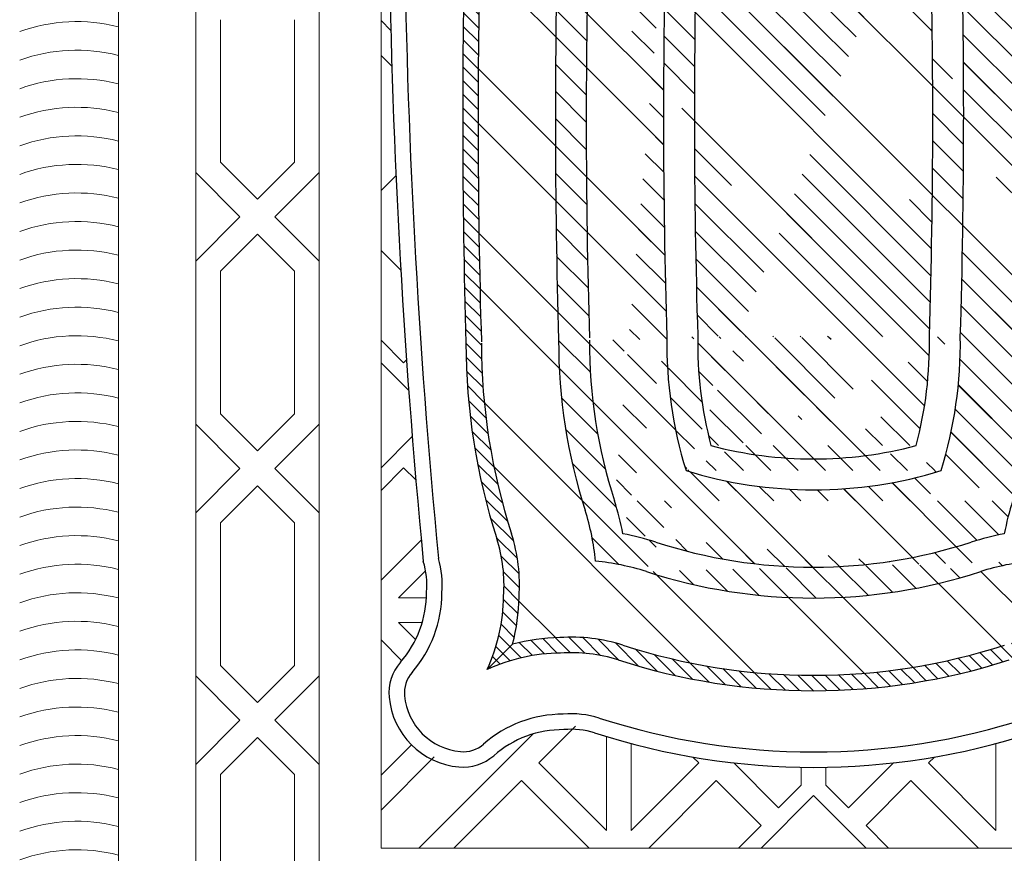
# Model space of a CAD drawing. Units: inches. Extents: x 3592 to 4861, y 1650 to 2243.
# Tile 7 of 30: x 4188 to 4207, y 1916 to 1932. Entities that reach past the tile are written whole.
import ezdxf

# ---------------------------------------------------------------- set-up
doc = ezdxf.new("R2010")
doc.units = ezdxf.units.IN
doc.layers.add('A-FURN', color=9, linetype='Continuous', lineweight=13)
doc.layers.add('RA-AP-01$0$INT', color=35, linetype='Continuous', lineweight=5)
for name, color, linetype in [('RA-AP-01$0$FURN', 3, 'Continuous'), ('RA-AP-01$0$WOOD', 64, 'Continuous'), ('RA-AP-02$0$FLPT', 30, 'Continuous')]:
    doc.layers.add(name, color=color, linetype=linetype)

# ---------------------------------------------------------------- blocks, each defined once
blk = doc.blocks.new('A$C67D63ADA')
at = {"layer": 'RA-AP-01$0$INT'}
for p, q in [((5.477240000007288, -6.923416270324413), (5.477239999992479, -6.363416270332882)), ((5.409652332498168, -6.525357395822982), (5.465926291497726, -6.525357395821494)), ((5.465926291497726, -6.525357395821494), (5.42221056274693, -6.569073124574231)), ((5.477239999997057, -6.536671104320128), (5.433524271246167, -6.580386833072967)), ((5.477239999998595, -6.59484772782809), (5.477239999997057, -6.536671104320128)), ((5.418357259801259, -6.565219821628732), (5.42221056274693, -6.569073124574231)), ((5.433524271246167, -6.580386833072966), (5.462612583000919, -6.609475144826422)), ((5.422140622500873, -6.591770481818769), (5.422210562747435, -6.591700541572205)), ((5.422210562747434, -6.591700541572205), (5.451298874502183, -6.62078885332566)), ((5.462612583000919, -6.609475144826422), (5.477239999998558, -6.594847727828128)), ((5.477239999998596, -6.59484772782809), (5.462612583000919, -6.609475144826423)), ((5.443298874502688, -6.64341627032368), (5.477239999998885, -6.609475144825973)), ((5.477239999998885, -6.609475144825973), (5.477240000000778, -6.677357395819498)), ((5.43667145750578, -6.635416270323993), (5.451298874503459, -6.620788853325663)), ((5.436671457504505, -6.635416270323988), (5.424977006995209, -6.635416270324199)), ((5.443298874502688, -6.64341627032368), (5.477240000000778, -6.677357395819498)), ((5.436671457504861, -6.651416270322137), (5.424977006995124, -6.651416270322447)), ((5.436671457506382, -6.65141627032399), (5.451298874503189, -6.666043687319815)), ((5.422210562749734, -6.695131999074563), (5.451298874503189, -6.666043687319815)), ((5.433524271248971, -6.706445707574319), (5.462612583002428, -6.677357395819569)), ((5.477240000000758, -6.691984812817247), (5.462612583002428, -6.677357395819567)), ((5.477240000000756, -6.691984812817247), (5.477240000001805, -6.750161436325209)), ((5.422140622500601, -6.695062058825432), (5.422210562749736, -6.695131999074563)), ((5.477240000001805, -6.750161436325209), (5.433524271248971, -6.706445707574317)), ((5.41835725979925, -6.721612719024712), (5.422210562750238, -6.717759416073553)), ((5.465926291502978, -6.761475144824349), (5.422210562750238, -6.717759416073553)), ((5.409652332496428, -6.761475144825365), (5.465926291502978, -6.761475144824349)), ((5.405096589281656, -6.777475144825446), (5.465926291503357, -6.777475144824348)), ((5.465926291503357, -6.777475144824348), (5.422210562752948, -6.821190873576702)), ((5.477240000002503, -6.788788853323175), (5.433524271252185, -6.832504582075438)), ((5.422210562752947, -6.821190873576701), (5.398502923497431, -6.797483234322237)), ((5.403480564853991, -6.825088292684419), (5.477240000004493, -6.898847727834922)), ((5.477240000004083, -6.876220310825392), (5.433524271252185, -6.832504582075438)), ((5.418311572313375, -6.889056385133678), (5.452671457504211, -6.923416270324519)), ((5.315298874504621, -6.912102561826071), (5.29779276232685, -6.894596449648303)), ((5.315298874504541, -6.893742340800933), (5.315298874504621, -6.912102561826071)), ((5.239087008341665, -6.900882970485501), (5.231181125499767, -6.908788853327399)), ((5.303985166005732, -6.923416270325152), (5.277960454425306, -6.89739155874473)), ((5.331298874504555, -6.896756776930311), (5.33129887450462, -6.912102561826093)), ((5.33129887450462, -6.912102561826093), (5.342348500618869, -6.901052935711843)), ((5.148671457508614, -6.923416270325409), (5.16329887450662, -6.908788853327405)), ((5.163298874506619, -6.908788853327405), (5.148671457508651, -6.923416270325372)), ((5.161430071025033, -6.906920049845819), (5.163298874506619, -6.908788853327405)), ((5.181214712172991, -6.905500432658874), (5.163298874506496, -6.923416270325372)), ((5.210977238572697, -6.903212383397972), (5.231181125500023, -6.923416270325749)), ((5.245808542497771, -6.923416270325402), (5.231181125499765, -6.908788853327399)), ((5.430044040505915, -6.923416270324613), (5.410388987144851, -6.903761216963554)), ((5.051867417002686, -6.92341627032501), (5.042215760114743, -6.913764613437067)), ((5.079181125501765, -6.912102561826092), (5.079336333743704, -6.911947353584153)), ((5.079181125501766, -6.911955542479179), (5.079181125501765, -6.912102561826092)), ((5.090494834000653, -6.923416270325169), (5.103286866518899, -6.91062423780692)), ((5.3426125830037, -6.923416270324986), (5.356067157599694, -6.909961695728989)), ((4.948123212422537, -6.917101600404618), (4.941808542500447, -6.923416270326709)), ((4.964435959500471, -6.923416270324652), (4.971407022751201, -6.916445207073921)), ((4.877240000006825, -6.923416270326986), (5.477240000007288, -6.923416270324413)), ((5.051867417002687, -6.923416270325013), (4.964435959500471, -6.923416270324652)), ((5.148671457508614, -6.923416270325408), (5.090494834000653, -6.923416270325169)), ((5.163298874506496, -6.923416270325372), (5.231181125500023, -6.923416270325749)), ((5.245808542497771, -6.923416270325401), (5.303985166005732, -6.923416270325152)), ((5.040068427124683, -6.963416270301689), (5.068754718630654, -6.992102561798438)), ((5.097441010136626, -6.963416270301689), (5.068754718630654, -6.992102561798438)), ((5.202896854259693, -6.963416270316853), (5.231583145756439, -6.992102561822827)), ((5.260269437262412, -6.963416270301053), (5.23158314575644, -6.992102561797802)), ((5.36572528138184, -6.963416270321417), (5.394411572878586, -6.99210256182739)), ((5.394411572878586, -6.99210256182739), (5.423097864384927, -6.963416270330275)), ((5.033441010127117, -6.979416270300584), (4.941240000005749, -6.979416270315998)), ((5.033441010127117, -6.979416270300584), (5.057441010133491, -7.00341627029924)), ((5.104068427130107, -6.979416270304665), (5.080068427127819, -7.00341627029924)), ((5.104068427130107, -6.979416270304665), (5.196269437263445, -6.979416270320077)), ((5.196269437263445, -6.979416270320077), (5.220269437255637, -7.003416270319991)), ((5.266896854262809, -6.979416270297111), (5.242896854253604, -7.003416270298604)), ((5.266896854262809, -6.979416270297111), (5.359097864373478, -6.979416270312523)), ((5.359097864373478, -6.979416270312523), (5.383097864377784, -7.003416270324554)), ((5.405725281375753, -7.003416270328198), (5.42972528138643, -6.979416270325234)), ((5.52192629150337, -6.97941627032422), (5.42972528138643, -6.979416270325234)), ((5.033441010139864, -7.027416270300586), (5.057441010133491, -7.00341627029924)), ((5.104068427125523, -7.027416270304664), (5.080068427127819, -7.00341627029924)), ((5.196269437247836, -7.027416270320077), (5.220269437255637, -7.003416270319991)), ((5.266896854244392, -7.027416270297113), (5.242896854253604, -7.003416270298604)), ((5.359097864382099, -7.027416270312525), (5.383097864377784, -7.003416270324554)), ((5.405725281375753, -7.003416270328198), (5.429725281365354, -7.027416270325517)), ((5.040068427138238, -7.043416270301689), (5.068754718634292, -7.014729978796407)), ((5.097441010123072, -7.043416270301689), (5.068754718627016, -7.014729978796407)), ((5.202896854247523, -7.043416270316853), (5.231583145752804, -7.014729978820797)), ((5.260269437248857, -7.043416270301053), (5.231583145752802, -7.01472997879577)), ((5.36572528136967, -7.043416270321417), (5.394411572874951, -7.014729978825361)), ((5.394411572874951, -7.014729978825361), (5.423097864372064, -7.043416270331702)), ((5.033441010139864, -7.027416270300586), (4.941240000013775, -7.027416270315999)), ((5.104068427125523, -7.027416270304664), (5.196269437247836, -7.027416270320077)), ((5.266896854244392, -7.027416270297113), (5.359097864382099, -7.027416270312525)), ((5.429725281365354, -7.027416270325517), (5.521926291510647, -7.027416270325517))]:
    blk.add_line(p, q, dxfattribs=at)
for points in [[(5.647240000006826, -6.243416270325369), (5.647240000006826, -7.09341627032537), (4.107240000006826, -7.093416270325372), (4.107240000006826, -6.19341627032537), (4.877240000006826, -6.19341627032537)], [(4.877240000006826, -6.19341627032537), (5.647240000006826, -6.19341627032537), (5.647240000006826, -7.09341627032537), (4.877240000006826, -7.09341627032537)], [(5.597240000006826, -6.243416270325369), (5.597240000006826, -7.04341627032537), (4.157240000006826, -7.043416270325372), (4.157240000006826, -6.243416270325369)], [(4.877240000006826, -6.32341627032537), (5.517240000006826, -6.32341627032537), (5.517240000006826, -6.963416270325371), (4.877240000006826, -6.963416270325371)]]:
    blk.add_lwpolyline(points, dxfattribs=at)
for centre, start in [((5.051601958963728, -7.120376270327977), 165.6974573627986), ((5.070081958960181, -7.120376270327977), 165.6974573627986), ((5.088561958964091, -7.120376270329249), 165.6974573621089), ((5.10704195896309, -7.120376270327067), 165.6974573632914), ((5.12552195896209, -7.120376270327067), 165.6974573632914), ((5.144001958965818, -7.12037627032834), 165.6974573626017), ((5.162481958964817, -7.12037627032743), 165.6974573630946), ((5.18096195896127, -7.12037627032743), 165.6974573630946), ((5.19944195896518, -7.120376270328703), 165.6974573624049), ((5.217921958963997, -7.120376270330159), 165.6974573616162), ((5.236401958960631, -7.120376270327794), 165.6974573628977), ((5.25488195896436, -7.120376270327977), 165.6974573627986), ((5.273361958963359, -7.120376270329249), 165.6974573621089), ((5.291841958964723, -7.120376270330522), 165.6974573614194), ((5.310321958963722, -7.12037627032834), 165.6974573626017), ((5.328801958964235, -7.120376270330886), 165.6974573612222), ((5.328801958965086, -7.120376270328522), 165.6974573625031), ((5.347281958963233, -7.120376270328703), 165.6974573624049), ((5.365761958962233, -7.120376270328703), 165.6974573624049), ((5.384241958965962, -7.120376270329977), 165.6974573617145), ((5.402721958964961, -7.120376270329067), 165.6974573622072), ((5.421201958961413, -7.120376270329067), 165.6974573622072), ((5.439681958965324, -7.120376270330341), 165.6974573615171), ((5.458161958964141, -7.120376270331796), 165.6974573607288), ((5.476641958960775, -7.120376270329431), 165.6974573620099), ((5.495121958964504, -7.120376270329613), 165.6974573619117), ((5.513601958963502, -7.120376270330886), 165.6974573612216), ((5.532081958964867, -7.12037627033216), 165.6974573605316), ((5.550561958963865, -7.120376270329977), 165.6974573617144), ((5.56904195896523, -7.120376270330159), 165.6974573616157), ((5.587521958961682, -7.120376270332524), 165.6974573603342)]:
    blk.add_arc(centre, 0.1091312342836184, start, 199.7961568705686, dxfattribs=at)
blk = doc.blocks.new('A$C09A87C41')
at = {"layer": 'RA-AP-01$0$WOOD'}
h = blk.add_hatch(dxfattribs=at)
h.set_pattern_fill('ANSI31', color=256, scale=0.05, style=0)
h.set_pattern_definition([(45, (0.7182879904584168, -11.54818755465011), (0.0044194173824159, -0.0044194173824159), [])])
edge = h.paths.add_edge_path()
edge.add_ellipse((5.006516613079209, -11.27459283286495), major_axis=(3.435359877543153, 3.435359877543153), ratio=0.9999999999999982, start_angle=403.3022422558093, end_angle=406.5486575131389, ccw=False)
edge.add_ellipse((5.150455045735207, -6.828790194879051), major_axis=(-0.2901946312779826, 0.2901946312779826), ratio=0.9999999999999875, start_angle=297.2093186994243, end_angle=314.9999999999731, ccw=False)
edge.add_ellipse((5.307117976013378, -6.343033378039902), major_axis=(-0.0707106781186454, 0.0707106781186455), ratio=0.9999999999999651, start_angle=116.7779839927149, end_angle=139.0873288843009)
edge.add_ellipse((5.312718414970339, -6.324818905441738), major_axis=(0.0834173982641243, 0.0834173982641243), ratio=0.9999999999999847, start_angle=225.741775187377, end_angle=249.5633269497028)
edge.add_line((5.361758401537698, -6.432112914518591), (5.345299417747169, -6.448571898309089))
edge.add_ellipse((5.312718414970311, -6.32481890544173), major_axis=(-0.0904884660759946, 0.0904884660759945), ratio=0.9999999999999644, start_angle=135.8720682536374, end_angle=149.7498089726665, ccw=False)
edge.add_ellipse((5.307117976013483, -6.343033378039922), major_axis=(-0.0777817459304867, 0.0777817459304867), ratio=0.9999999999999941, start_angle=117.45144083316339, end_angle=138.9346900893823, ccw=False)
edge.add_ellipse((5.150455045735208, -6.82879019487905), major_axis=(0.2831235634661059, 0.2831235634661059), ratio=0.9999999999999859, start_angle=27.03507540014952, end_angle=44.9867285887044)
edge.add_ellipse((5.006516315412802, -11.27459997798134), major_axis=(-3.428298916554014, 3.428298916554014), ratio=0.9999999999999971, start_angle=-46.70235550375367, end_angle=-43.44815559494434)
edge.add_ellipse((4.743915471599394, -11.2745999779814), major_axis=(3.428298916553931, 3.42829891655393), ratio=0.9999999999999994, start_angle=43.44815559494427, end_angle=46.70235550375375)
edge.add_ellipse((4.599976741276995, -6.828790194879051), major_axis=(0.2831235634661173, 0.2831235634661172), ratio=0.9999999999999861, start_angle=45.01327141129749, end_angle=62.96492459984043)
edge.add_ellipse((4.443313810998718, -6.343033378039922), major_axis=(0.0777817459304893, 0.0777817459304893), ratio=0.9999999999999873, start_angle=221.0653099106178, end_angle=242.54855916687399, ccw=False)
edge.add_ellipse((4.437713372041892, -6.32481890544173), major_axis=(0.0904884660759951, 0.0904884660759951), ratio=0.9999999999999603, start_angle=210.2501910273332, end_angle=224.1279317463614, ccw=False)
edge.add_line((4.405132369265034, -6.448571898309089), (4.388673385474508, -6.432112914518594))
edge.add_ellipse((4.43771337204186, -6.324818905441737), major_axis=(0.0834173982641232, 0.0834173982641232), ratio=0.9999999999999797, start_angle=200.4366730503009, end_angle=224.2582248126243)
edge.add_ellipse((4.443313810998827, -6.343033378039902), major_axis=(-0.0707106781186382, 0.0707106781186382), ratio=0.9999999999999952, start_angle=130.9126711156974, end_angle=153.2220160072772)
edge.add_ellipse((4.599976741276995, -6.828790194879051), major_axis=(-0.2901946312779718, 0.2901946312779718), ratio=0.9999999999999895, start_angle=315.0000000000233, end_angle=332.7906813005773, ccw=False)
edge.add_ellipse((4.743915173933024, -11.27459283286497), major_axis=(-3.435359877543123, 3.435359877543123), ratio=0.9999999999999991, start_angle=313.451342486861, end_angle=316.69775774419077, ccw=False)
edge = h.paths.add_edge_path()
edge.add_ellipse((4.299593848995801, -6.48675334004306), major_axis=(-0.0707106781186556, 0.0707106781186556), ratio=0.9999999999999859, start_angle=206.7779839906583, end_angle=229.0873288838364)
edge.add_ellipse((4.281379376397651, -6.481152901086075), major_axis=(-0.0834173982641623, 0.0834173982641623), ratio=0.9999999999999754, start_angle=225.7417751869729, end_angle=249.5633269497573)
edge.add_line((4.388673385474506, -6.432112914518592), (4.405132369265034, -6.448571898309089))
edge.add_ellipse((4.281379376397657, -6.481152901086004), major_axis=(-0.0904884660760182, 0.0904884660760182), ratio=0.9999999999999957, start_angle=225.8720682533453, end_angle=239.7498089726896, ccw=False)
edge.add_ellipse((4.299593848995796, -6.486753340043026), major_axis=(0.0777817459305317, 0.0777817459305317), ratio=0.9999999999999891, start_angle=297.4514408381613, end_angle=318.9346900891407, ccw=False)
edge.add_ellipse((4.785350665835052, -6.643416270320893), major_axis=(0.2831235634661102, 0.2831235634661102), ratio=0.9999999999999978, start_angle=117.0350753988375, end_angle=152.9649246009711)
edge.add_ellipse((4.299593848995777, -6.800079200598784), major_axis=(-0.0777817459305426, 0.0777817459305426), ratio=0.9999999999999973, start_angle=221.0653099111909, end_angle=242.5485591625442, ccw=False)
edge.add_ellipse((4.281379376397679, -6.805679639555494), major_axis=(-0.0904884660760244, 0.0904884660760244), ratio=0.9999999999999076, start_angle=210.2501910270576, end_angle=224.1279317467988, ccw=False)
edge.add_line((4.405132369264926, -6.838260642332959), (4.388673385474263, -6.854719626123697))
edge.add_ellipse((4.281379376397679, -6.80567963955562), major_axis=(0.0834173982641642, 0.0834173982641642), ratio=0.9999999999999609, start_angle=290.4366730499258, end_angle=314.2582248131156)
edge.add_ellipse((4.299593848995804, -6.800079200598786), major_axis=(-0.0707106781186612, 0.0707106781186612), ratio=0.999999999999977, start_angle=220.9126711163551, end_angle=243.222016008517)
edge.add_ellipse((4.785350665835053, -6.643416270320894), major_axis=(0.2901946312779783, 0.2901946312779783), ratio=0.9999999999999984, start_angle=117.2093186999746, end_angle=152.7906813002342, ccw=False)
edge = h.paths.add_edge_path()
edge.add_ellipse((4.743915471599392, -2.012232562660299), major_axis=(3.428298916553894, 3.428298916553894), ratio=0.9999999999999992, start_angle=223.2976444962459, end_angle=226.5518444050561)
edge.add_ellipse((5.006516315412771, -2.012232562660296), major_axis=(3.428298916553752, 3.428298916553752), ratio=0.9999999999999971, start_angle=223.448155594945, end_angle=226.7023555037531)
edge.add_ellipse((5.150455045735209, -6.458042345762599), major_axis=(0.283123563466111, 0.283123563466111), ratio=0.999999999999996, start_angle=225.0132714112834, end_angle=242.9649246011241)
edge.add_ellipse((5.30711797601273, -6.94379916260194), major_axis=(0.0777817459305174, 0.0777817459305174), ratio=0.9999999999999873, start_angle=401.06530991071423, end_angle=422.548559161793, ccw=False)
edge.add_ellipse((5.312718414969516, -6.962013635200094), major_axis=(0.0904884660760023, 0.0904884660760023), ratio=0.9999999999999566, start_angle=390.2501910269164, end_angle=404.12793174642553, ccw=False)
edge.add_line((5.345299417747278, -6.838260642332959), (5.361758401537942, -6.854719626123698))
edge.add_ellipse((5.312718414969516, -6.962013635200098), major_axis=(0.0834173982641439, 0.0834173982641439), ratio=0.9999999999999785, start_angle=20.43667304973462, end_angle=44.25822481258737)
edge.add_ellipse((5.307117976012772, -6.943799162601948), major_axis=(-0.0707106781186618, 0.0707106781186618), ratio=0.999999999999977, start_angle=-49.08732888421749, end_angle=-26.77798399064677)
edge.add_ellipse((5.150455045735209, -6.458042345762597), major_axis=(0.2901946312779783, 0.2901946312779783), ratio=0.9999999999999957, start_angle=225.0000000000273, end_angle=242.7906812999824, ccw=False)
edge.add_ellipse((5.006516613079198, -2.012239707776725), major_axis=(3.43535987754352, 3.43535987754352), ratio=0.999999999999996, start_angle=223.4513424868609, end_angle=226.697757744191, ccw=False)
edge.add_ellipse((4.743915173933023, -2.012239707776712), major_axis=(3.435359877543229, 3.435359877543229), ratio=0.9999999999999998, start_angle=223.3022422558095, end_angle=226.5486575131387, ccw=False)
edge.add_ellipse((4.599976741276995, -6.458042345762597), major_axis=(0.2901946312779746, 0.2901946312779748), ratio=0.9999999999999964, start_angle=207.2093187000184, end_angle=224.9999999999795, ccw=False)
edge.add_ellipse((4.443313810999427, -6.943799162601947), major_axis=(-0.070710678118668, 0.070710678118668), ratio=0.9999999999999838, start_angle=-63.22201600935903, end_angle=-40.9126711157662)
edge.add_ellipse((4.437713372042683, -6.962013635200099), major_axis=(0.0834173982641484, 0.0834173982641484), ratio=0.9999999999999729, start_angle=45.74177518742643, end_angle=69.56332695026246)
edge.add_line((4.388673385474263, -6.854719626123697), (4.405132369264926, -6.838260642332958))
edge.add_ellipse((4.437713372042681, -6.962013635200094), major_axis=(0.0904884660760224, 0.0904884660760225), ratio=0.9999999999999282, start_angle=405.87206825357924, end_angle=419.7498089730807, ccw=False)
edge.add_ellipse((4.443313810999475, -6.94379916260194), major_axis=(-0.0777817459305165, 0.0777817459305165), ratio=0.9999999999999927, start_angle=297.4514408382556, end_angle=318.93469008929503, ccw=False)
edge.add_ellipse((4.599976741276995, -6.458042345762597), major_axis=(0.2831235634661077, 0.2831235634661077), ratio=0.9999999999999937, start_angle=207.0350753988627, end_angle=224.9867285886981)
edge = h.paths.add_edge_path()
edge.add_ellipse((5.450837938016399, -6.800079200598789), major_axis=(-0.0707106781186565, 0.0707106781186565), ratio=0.9999999999999875, start_angle=26.77798399147072, end_angle=49.08732888364846)
edge.add_ellipse((5.469052410614524, -6.80567963955562), major_axis=(0.0834173982641601, 0.0834173982641601), ratio=0.9999999999999984, start_angle=135.7417751868887, end_angle=159.563326950074)
edge.add_line((5.36175840153794, -6.854719626123697), (5.345299417747278, -6.838260642332959))
edge.add_ellipse((5.469052410614523, -6.805679639555488), major_axis=(0.0904884660760307, 0.0904884660760307), ratio=0.9999999999999984, start_angle=135.8720682531977, end_angle=149.7498089729454, ccw=False)
edge.add_ellipse((5.450837938016426, -6.800079200598787), major_axis=(0.0777817459305426, 0.0777817459305427), ratio=0.9999999999999968, start_angle=117.4514408374904, end_angle=138.9346900888003, ccw=False)
edge.add_ellipse((4.965081121177151, -6.643416270320895), major_axis=(-0.2831235634661119, 0.2831235634661119), ratio=0.9999999999999992, start_angle=207.0350753990193, end_angle=242.9649246011595)
edge.add_ellipse((5.450837938016407, -6.486753340043026), major_axis=(0.0777817459305285, 0.0777817459305285), ratio=0.9999999999999747, start_angle=131.0653099108597, end_angle=152.5485591618505, ccw=False)
edge.add_ellipse((5.469052410614547, -6.481152901086004), major_axis=(0.09048846607603, 0.09048846607603), ratio=0.9999999999999619, start_angle=120.25019102731059, end_angle=134.1279317466551, ccw=False)
edge.add_line((5.345299417747169, -6.448571898309089), (5.361758401537697, -6.432112914518592))
edge.add_ellipse((5.469052410614551, -6.481152901086075), major_axis=(-0.0834173982641603, 0.0834173982641603), ratio=0.9999999999999998, start_angle=20.43667305024269, end_angle=44.25822481302925)
edge.add_ellipse((5.450837938016403, -6.486753340043062), major_axis=(-0.0707106781186603, 0.0707106781186603), ratio=0.9999999999999737, start_angle=40.91267111616517, end_angle=63.22201600943157)
edge.add_ellipse((4.965081121177149, -6.643416270320895), major_axis=(0.2901946312779771, 0.2901946312779771), ratio=0.9999999999999992, start_angle=297.2093186997686, end_angle=332.7906813000034, ccw=False)
h = blk.add_hatch(dxfattribs=at)
h.set_pattern_fill('ANSI32', color=256, scale=0.2, style=0)
h.set_pattern_definition([(45, (0.7182879904584168, -11.54818755465011), (0.0530330085889911, -0.0530330085889911), []), (45, (0.7182879904584168, -11.51283221565011), (0.0530330085889911, -0.0530330085889911), [])])
edge = h.paths.add_edge_path()
edge.add_ellipse((5.15045504573521, -6.82879019487905), major_axis=(-0.2831235634661157, 0.2831235634661156), ratio=0.9999999999999889, start_angle=297.21454354460053, end_angle=314.98672858870884, ccw=False)
edge.add_ellipse((5.307117976013485, -6.343033378039922), major_axis=(-0.0777817459304881, 0.0777817459304881), ratio=0.9999999999999928, start_angle=116.7981781115797, end_angle=138.9346900893818)
edge.add_ellipse((5.312718414970311, -6.32481890544173), major_axis=(-0.0904884660759946, 0.0904884660759946), ratio=0.9999999999999658, start_angle=135.8720682536378, end_angle=149.7498089726664)
edge.add_ellipse((5.469052410614547, -6.481152901086004), major_axis=(0.0904884660760303, 0.0904884660760302), ratio=0.9999999999999603, start_angle=120.2501910273106, end_angle=134.1279317466551)
edge.add_ellipse((5.450837938016407, -6.486753340043026), major_axis=(-0.0777817459305327, 0.0777817459305327), ratio=0.9999999999999915, start_angle=41.06530991085969, end_angle=63.20182189333976)
edge.add_ellipse((4.965081121177151, -6.643416270320894), major_axis=(-0.2831235634661133, 0.2831235634661133), ratio=0.9999999999999984, start_angle=207.214543545815, end_angle=242.7854564539869, ccw=False)
edge.add_ellipse((5.450837938016426, -6.800079200598786), major_axis=(0.0777817459305424, 0.0777817459305424), ratio=0.9999999999999962, start_angle=116.7981781073729, end_angle=138.9346900888086)
edge.add_ellipse((5.469052410614524, -6.805679639555493), major_axis=(0.0904884660760289, 0.0904884660760289), ratio=0.9999999999999841, start_angle=135.872068253202, end_angle=149.7498089729424)
edge.add_ellipse((5.312718414969522, -6.962013635200094), major_axis=(-0.0904884660760224, 0.0904884660760225), ratio=0.9999999999999282, start_angle=-59.7498089730807, end_angle=-45.87206825357926)
edge.add_ellipse((5.307117976012728, -6.94379916260194), major_axis=(0.0777817459305181, 0.0777817459305181), ratio=0.9999999999999861, start_angle=41.06530991070497, end_angle=63.20182189334603)
edge.add_ellipse((5.150455045735208, -6.458042345762599), major_axis=(0.2831235634661146, 0.2831235634661146), ratio=0.9999999999999907, start_angle=225.013271411291, end_angle=242.7854564539341, ccw=False)
edge.add_ellipse((5.006516315412806, -2.012232562660296), major_axis=(3.428298916554143, 3.428298916554143), ratio=0.9999999999999941, start_angle=223.4481555949448, end_angle=226.7023555037533, ccw=False)
edge.add_ellipse((4.743915471599424, -2.012232562660299), major_axis=(3.428298916554168, 3.428298916554171), ratio=0.9999999999999991, start_angle=223.2976444962462, end_angle=226.551844405056, ccw=False)
edge.add_ellipse((4.599976741276996, -6.458042345762597), major_axis=(0.2831235634661098, 0.2831235634661098), ratio=0.9999999999999973, start_angle=207.2145435460398, end_angle=224.9867285887048, ccw=False)
edge.add_ellipse((4.443313810999473, -6.94379916260194), major_axis=(-0.0777817459305183, 0.0777817459305183), ratio=0.9999999999999823, start_angle=-63.2018218932521, end_angle=-41.06530991071377)
edge.add_ellipse((4.437713372042686, -6.962013635200094), major_axis=(-0.0904884660760028, 0.0904884660760028), ratio=0.9999999999999504, start_angle=-44.12793174642511, end_angle=-30.25019102691602)
edge.add_ellipse((4.281379376397679, -6.80567963955549), major_axis=(-0.0904884660760215, 0.0904884660760215), ratio=0.9999999999999245, start_angle=210.2501910270558, end_angle=224.1279317467963)
edge.add_ellipse((4.299593848995777, -6.800079200598786), major_axis=(0.077781745930539, 0.077781745930539), ratio=0.999999999999963, start_angle=311.0653099111909, end_angle=333.2018218926339)
edge.add_ellipse((4.785350665835052, -6.643416270320894), major_axis=(0.2831235634661089, 0.2831235634661091), ratio=0.9999999999999989, start_angle=117.21454354600829, end_angle=152.7854564541833, ccw=False)
edge.add_ellipse((4.299593848995796, -6.486753340043026), major_axis=(0.077781745930533, 0.077781745930533), ratio=0.9999999999999792, start_angle=296.7981781066777, end_angle=318.9346900891398)
edge.add_ellipse((4.281379376397657, -6.481152901086003), major_axis=(-0.0904884660760217, 0.0904884660760217), ratio=0.9999999999999742, start_angle=225.872068253344, end_angle=239.7498089726891)
edge.add_ellipse((4.437713372041892, -6.32481890544173), major_axis=(0.090488466075997, 0.090488466075997), ratio=0.9999999999999756, start_angle=210.2501910273331, end_angle=224.1279317463622)
edge.add_ellipse((4.44331381099872, -6.343033378039923), major_axis=(0.0777817459304873, 0.0777817459304872), ratio=0.9999999999999861, start_angle=221.0653099106177, end_angle=243.2018218883976)
edge.add_ellipse((4.599976741276995, -6.828790194879051), major_axis=(-0.2831235634661067, 0.2831235634661067), ratio=0.9999999999999895, start_angle=315.01327141129775, end_angle=332.78545645540567, ccw=False)
edge.add_ellipse((4.743915471599392, -11.2745999779814), major_axis=(-3.428298916553902, 3.428298916553902), ratio=0.9999999999999984, start_angle=313.4481555949443, end_angle=316.7023555037538, ccw=False)
edge.add_ellipse((5.006516315412786, -11.27459997798134), major_axis=(-3.428298916554052, 3.428298916554052), ratio=1, start_angle=313.29764449624645, end_angle=316.5518444050555, ccw=False)
edge = h.paths.add_edge_path(flags=16)
edge.add_ellipse((4.745320840887742, -11.27459782170807), major_axis=(3.392940520945516, 3.392940520945516), ratio=1, start_angle=43.44876692339471, end_angle=46.71249975461917)
edge.add_ellipse((4.599976741276995, -6.828790194878992), major_axis=(-0.2477682244067734, 0.2477682244067734), ratio=0.9999999999999911, start_angle=-45.31868720933983, end_angle=-27.00912183057358)
edge.add_ellipse((4.443313810998828, -6.343033378039872), major_axis=(0.1131370849898469, 0.1131370849898469), ratio=0.9999999999999724, start_angle=230.5682590208478, end_angle=242.6218359751805, ccw=False)
edge.add_ellipse((4.299593848995757, -6.486753340043112), major_axis=(-0.1131370849898624, 0.1131370849898624), ratio=0.9999999999999953, start_angle=207.3781640250758, end_angle=219.4317409792351, ccw=False)
edge.add_ellipse((4.78535066583505, -6.643416270320884), major_axis=(0.2477682244067863, 0.2477682244067863), ratio=0.9999999999999974, start_angle=117.0091218305267, end_angle=152.9908781690427)
edge.add_ellipse((4.299593848995773, -6.800079200598856), major_axis=(0.1131370849898833, 0.1131370849898833), ratio=0.9999999999999682, start_angle=320.56825902084296, end_angle=332.62183597593753, ccw=False)
edge.add_ellipse((4.443313810999473, -6.943799162601939), major_axis=(0.1131370849898351, 0.1131370849898351), ratio=0.9999999999999213, start_angle=387.3781640246361, end_angle=399.43174097937606, ccw=False)
edge.add_ellipse((4.599976741276996, -6.458042345762606), major_axis=(0.2477682244067743, 0.2477682244067742), ratio=0.99999999999999, start_angle=207.0091218307682, end_angle=225.3186872093523)
edge.add_ellipse((4.745320840887777, -2.012234718933553), major_axis=(-3.392940520945741, 3.392940520945741), ratio=0.9999999999999992, start_angle=133.2875002453813, end_angle=136.5512330766047)
edge.add_ellipse((5.005110946124445, -2.012234718933546), major_axis=(3.392940520945412, 3.392940520945411), ratio=0.9999999999999989, start_angle=223.4487669233947, end_angle=226.7124997546191)
edge.add_ellipse((5.150455045735207, -6.458042345762608), major_axis=(-0.2477682244067739, 0.2477682244067739), ratio=0.9999999999999966, start_angle=134.6813127906568, end_angle=152.9908781692236)
edge.add_ellipse((5.30711797601273, -6.943799162601939), major_axis=(-0.1131370849898406, 0.1131370849898406), ratio=0.9999999999999811, start_angle=320.568259020624, end_angle=332.62183597538194, ccw=False)
edge.add_ellipse((5.45083793801643, -6.800079200598855), major_axis=(0.113137084989895, 0.113137084989895), ratio=0.999999999999955, start_angle=117.3781640240419, end_angle=129.4317409791577, ccw=False)
edge.add_ellipse((4.965081121177152, -6.643416270320884), major_axis=(0.2477682244067847, 0.2477682244067847), ratio=0.9999999999999992, start_angle=297.0091218309669, end_angle=332.990878169475)
edge.add_ellipse((5.450837938016447, -6.486753340043118), major_axis=(-0.1131370849898789, 0.1131370849898789), ratio=0.9999999999999342, start_angle=50.56825902076281, end_angle=62.62183597491821, ccw=False)
edge.add_ellipse((5.30711797601337, -6.34303337803987), major_axis=(0.1131370849898374, 0.1131370849898374), ratio=0.9999999999999493, start_angle=207.3781640247929, end_angle=219.4317409791543, ccw=False)
edge.add_ellipse((5.150455045735204, -6.828790194878992), major_axis=(-0.2477682244067807, 0.2477682244067808), ratio=0.9999999999999934, start_angle=-62.99087816941401, end_angle=-44.68131279065508)
edge.add_ellipse((5.005110946124442, -11.27459782170805), major_axis=(3.392940520945543, 3.392940520945543), ratio=0.9999999999999974, start_angle=43.28750024538099, end_angle=46.55123307660507)
edge = h.paths.add_edge_path(flags=0)
edge.add_ellipse((4.745321446260899, -11.27461227828643), major_axis=(3.378818834290158, 3.378818834290157), ratio=0.9999999999999996, start_angle=43.44228925150885, end_angle=46.72161971502517)
edge.add_ellipse((4.599976741276998, -6.828790194878991), major_axis=(-0.2336260887830454, 0.2336260887830454), ratio=0.9999999999999974, start_angle=-45.30974264369766, end_angle=-26.99844483641433)
edge.add_ellipse((4.443313810998811, -6.343033378039858), major_axis=(0.1272792206135962, 0.1272792206135962), ratio=0.9999999999999403, start_angle=235.6264990356023, end_angle=242.6432427499436, ccw=False)
edge.add_ellipse((4.299593848995773, -6.486753340043007), major_axis=(0.1272792206136285, 0.1272792206136286), ratio=0.9999999999999204, start_angle=297.35675724967757, end_angle=304.3735009644582, ccw=False)
edge.add_ellipse((4.785350665835048, -6.643416270320905), major_axis=(0.2336260887830504, 0.2336260887830504), ratio=0.9999999999999921, start_angle=116.998444836676, end_angle=153.0015551636886)
edge.add_ellipse((4.299593848995741, -6.800079200598703), major_axis=(-0.1272792206136906, 0.1272792206136906), ratio=0.9999999999996289, start_angle=235.62649903554922, end_angle=242.64324274961962, ccw=False)
edge.add_ellipse((4.443313810999469, -6.943799162601998), major_axis=(-0.1272792206136219, 0.1272792206136219), ratio=0.9999999999999658, start_angle=297.3567572500489, end_angle=304.3735009646209, ccw=False)
edge.add_ellipse((4.599976741276995, -6.458042345762605), major_axis=(0.2336260887830445, 0.2336260887830445), ratio=0.9999999999999957, start_angle=206.9984448365414, end_angle=225.3097426436968)
edge.add_ellipse((4.745321446260921, -2.012220262355212), major_axis=(3.378818834290089, 3.378818834290088), ratio=0.9999999999999994, start_angle=223.2783802849744, end_angle=226.5577107484907)
edge.add_ellipse((5.005110340751275, -2.012220262355198), major_axis=(3.378818834290274, 3.378818834290274), ratio=0.9999999999999992, start_angle=223.4422892515091, end_angle=226.7216197150253)
edge.add_ellipse((5.150455045735206, -6.458042345762609), major_axis=(0.2336260887830463, 0.2336260887830463), ratio=0.9999999999999937, start_angle=224.6902573562994, end_angle=243.0015551634542)
edge.add_ellipse((5.30711797601273, -6.943799162602), major_axis=(-0.1272792206135949, 0.1272792206135949), ratio=0.9999999999997138, start_angle=325.62649903537766, end_angle=332.6432427499585, ccw=False)
edge.add_ellipse((5.450837938016461, -6.800079200598699), major_axis=(-0.1272792206135936, 0.1272792206135936), ratio=0.999999999999666, start_angle=27.356757250387716, end_angle=34.37350096445232, ccw=False)
edge.add_ellipse((4.965081121177155, -6.643416270320904), major_axis=(0.23362608878305, 0.23362608878305), ratio=0.9999999999999992, start_angle=296.9984448363078, end_angle=333.0015551633219)
edge.add_ellipse((5.450837938016428, -6.486753340043003), major_axis=(0.1272792206136045, 0.1272792206136045), ratio=0.9999999999999529, start_angle=145.6264990355431, end_angle=152.6432427503271, ccw=False)
edge.add_ellipse((5.307117976013396, -6.34303337803986), major_axis=(0.1272792206135615, 0.1272792206135615), ratio=0.9999999999996925, start_angle=207.3567572500474, end_angle=214.3735009643965, ccw=False)
edge.add_ellipse((5.150455045735208, -6.828790194878991), major_axis=(-0.2336260887830484, 0.2336260887830485), ratio=0.9999999999999953, start_angle=-63.00155516358085, end_angle=-44.69025735630093)
edge.add_ellipse((5.005110340751286, -11.27461227828636), major_axis=(-3.378818834290266, 3.378818834290266), ratio=0.9999999999999998, start_angle=-46.72161971502535, end_angle=-43.44228925150914)
edge = h.paths.add_edge_path(flags=0)
edge.add_ellipse((4.747128261062206, -11.27459926241731), major_axis=(-3.343445075648777, 3.343445075648777), ratio=0.9999999999999991, start_angle=-46.55229325491085, end_angle=-43.26504392007965)
edge.add_ellipse((4.599976741277094, -6.828790194878977), major_axis=(0.198270749723715, 0.198270749723715), ratio=0.999999999999988, start_angle=44.18347671010175, end_angle=62.12936993332099)
edge.add_ellipse((4.785350665835048, -6.643416270320889), major_axis=(0.198270749723727, 0.198270749723727), ratio=0.9999999999999971, start_angle=117.8706300667295, end_angle=152.1293699332338)
edge.add_ellipse((4.599976741276998, -6.458042345762598), major_axis=(0.1982707497237202, 0.1982707497237202), ratio=0.9999999999999882, start_angle=207.8706300666892, end_angle=225.8165232899116)
edge.add_ellipse((4.747128261062279, -2.01223327822427), major_axis=(-3.343445075648579, 3.34344507564858), ratio=0.9999999999999984, start_angle=133.2650439200784, end_angle=136.5522932549098)
edge.add_ellipse((5.003303525949927, -2.012233278224277), major_axis=(-3.343445075648679, 3.343445075648679), ratio=0.9999999999999996, start_angle=133.4477067450899, end_angle=136.7349560799216)
edge.add_ellipse((5.150455045735204, -6.458042345762598), major_axis=(-0.1982707497237223, 0.1982707497237223), ratio=0.9999999999999994, start_angle=134.1834767100914, end_angle=152.1293699333112)
edge.add_ellipse((4.965081121177155, -6.643416270320892), major_axis=(0.1982707497237268, 0.1982707497237267), ratio=0.9999999999999987, start_angle=297.8706300667671, end_angle=332.1293699332712)
edge.add_ellipse((5.150455045735109, -6.828790194878977), major_axis=(0.1982707497237106, 0.1982707497237105), ratio=0.9999999999999982, start_angle=27.87063006667902, end_angle=45.8165232898948)
edge.add_ellipse((5.00330352595001, -11.2745992624173), major_axis=(3.343445075648743, 3.343445075648743), ratio=0.9999999999999996, start_angle=43.26504392007961, end_angle=46.55229325491089)
edge = h.paths.add_edge_path(flags=0)
edge.add_ellipse((4.747685770081003, -11.27459857725902), major_axis=(3.329301968186143, 3.329301968186141), ratio=0.9999999999999989, start_angle=43.44789769190167, end_angle=46.74269456932172)
edge.add_ellipse((4.599976741277087, -6.828790194878972), major_axis=(-0.1841286140999701, 0.1841286140999702), ratio=0.9999999999999841, start_angle=-45.99531238101485, end_angle=-30.22398030679106)
edge.add_ellipse((4.785350665835029, -6.643416270320906), major_axis=(0.1841286140999794, 0.1841286140999793), ratio=0.9999999999999998, start_angle=120.2239803068321, end_angle=149.7760196931203)
edge.add_ellipse((4.599976741276998, -6.458042345762589), major_axis=(0.1841286140999956, 0.1841286140999956), ratio=0.9999999999999953, start_angle=210.2239803068005, end_angle=225.9953123810239)
edge.add_ellipse((4.747685770081015, -2.012233963382593), major_axis=(-3.329301968186209, 3.32930196818621), ratio=0.9999999999999991, start_angle=133.2573054306775, end_angle=136.5521023080975)
edge.add_ellipse((5.002746016931159, -2.012233963382618), major_axis=(-3.329301968186245, 3.329301968186245), ratio=0.9999999999999984, start_angle=133.447897691902, end_angle=136.7426945693227)
edge.add_ellipse((5.150455045735208, -6.458042345762592), major_axis=(-0.1841286140999912, 0.1841286140999912), ratio=0.9999999999999873, start_angle=134.0046876189747, end_angle=149.7760196931988)
edge.add_ellipse((4.965081121177172, -6.643416270320907), major_axis=(-0.1841286140999788, 0.1841286140999788), ratio=0.9999999999999968, start_angle=210.2239803068796, end_angle=239.7760196931682)
edge.add_ellipse((5.150455045735117, -6.82879019487897), major_axis=(0.1841286140999714, 0.1841286140999713), ratio=0.9999999999999896, start_angle=30.22398030679139, end_angle=45.99531238102014)
edge.add_ellipse((5.002746016931209, -11.274598577259), major_axis=(3.329301968186158, 3.329301968186158), ratio=1, start_angle=43.25730543067866, end_angle=46.5521023080979)
h = blk.add_hatch(dxfattribs=at)
h.set_pattern_fill('ANSI31', color=256, scale=0.1, style=0)
h.set_pattern_definition([(45, (0.7182879904584168, -11.54818755465011), (0.0088388347648318, -0.0088388347648318), [])])
edge = h.paths.add_edge_path(flags=16)
edge.add_arc((4.965081121177173, -6.643416270320907), 0.2603971832811541, 345.2239803068796, 374.7760196931681)
edge.add_arc((4.965081121177173, -6.643416270320907), 0.2603971832811541, -14.776019693120418, 14.77601969316811, ccw=False)
edge = h.paths.add_edge_path(flags=16)
edge.add_arc((4.785350665835029, -6.643416270320907), 0.2603971832811541, 165.223980306832, 194.7760196931204)
edge.add_arc((4.785350665835029, -6.643416270320907), 0.2603971832811541, 165.223980306832, 194.7760196931204, ccw=False)
edge = h.paths.add_edge_path(flags=0)
edge.add_arc((4.785350665835029, -6.643416270320907), 0.2603971832811541, 165.223980306832, 194.7760196931204)
edge.add_arc((4.785350665835029, -6.643416270320907), 0.2603971832811541, 165.223980306832, 194.7760196931204, ccw=False)
edge = h.paths.add_edge_path(flags=0)
edge.add_arc((4.785350665835029, -6.643416270320907), 0.2603971832811541, 165.223980306832, 194.7760196931204)
edge.add_arc((4.785350665835029, -6.643416270320907), 0.2603971832811541, 165.223980306832, 194.7760196931204, ccw=False)
edge = h.paths.add_edge_path(flags=0)
edge.add_arc((4.785350665835029, -6.643416270320907), 0.2603971832811541, 165.223980306832, 194.7760196931204)
edge.add_arc((4.785350665835029, -6.643416270320907), 0.2603971832811541, 165.223980306832, 194.7760196931204, ccw=False)
edge = h.paths.add_edge_path(flags=0)
edge.add_arc((4.785350665835029, -6.643416270320907), 0.2603971832811541, 165.223980306832, 194.7760196931204)
edge.add_arc((4.785350665835029, -6.643416270320907), 0.2603971832811541, 165.223980306832, 194.7760196931204, ccw=False)
edge = h.paths.add_edge_path(flags=0)
edge.add_arc((4.785350665835029, -6.643416270320907), 0.2603971832811541, 165.223980306832, 194.7760196931204)
edge.add_arc((4.785350665835029, -6.643416270320907), 0.2603971832811541, 165.223980306832, 194.7760196931204, ccw=False)
edge = h.paths.add_edge_path(flags=0)
edge.add_arc((4.785350665835029, -6.643416270320907), 0.2603971832811541, 165.223980306832, 194.7760196931204)
edge.add_arc((4.785350665835029, -6.643416270320907), 0.2603971832811541, 165.223980306832, 194.7760196931204, ccw=False)
edge = h.paths.add_edge_path()
edge.add_arc((5.30711797601273, -6.943799162601939), 0.1599999999999918, 95.56825902062381, 107.6218359753744)
edge.add_arc((5.150455045735207, -6.458042345762605), 0.3503971832811637, 269.6813127906517, 287.9908781692269)
edge.add_arc((5.307117976013371, -6.34303337803987), 0.1599999999999917, 252.3781640232651, 264.4317409791539)
edge.add_arc((4.965081121177153, -6.643416270320884), 0.3503971832811761, 342.0091218309644, 377.9908781694648)
edge.add_arc((5.005110946124438, -2.012234718933557), 4.798342501046485, 268.4423197280547, 271.7124997546188)
edge.add_arc((5.150455045735207, -6.828790194878991), 0.3503971832811637, 72.00912183077308, 90.31868720934834)
edge.add_arc((5.005110340751293, -2.012220262355208), 4.778371420254705, 268.433225420277, 271.7034061068158)
edge.add_arc((5.150455045735207, -6.828790194878991), 0.3303971832811637, 72.00912183077308, 90.31868720934834)
edge.add_arc((5.005110340751291, -11.27461227828638), 4.7783714202547, 88.29659389318418, 91.5667745797229)
edge.add_arc((5.450837938016446, -6.486753340043115), 0.1600000000000254, 185.5682590207637, 197.6218359749416)
edge.add_arc((5.450837938016429, -6.800079200598855), 0.1600000000000541, 162.3781640240467, 174.4317409791574)
edge.add_arc((5.307117976012735, -6.943799162601998), 0.1800000000000505, 100.6264990353792, 107.6432427499818)
edge.add_arc((5.307117976013394, -6.343033378039859), 0.1800000000000069, 252.3567572486067, 259.3735009643972)
edge.add_arc((5.45083793801643, -6.486753340043007), 0.1800000000000424, 190.6264990355417, 197.6432427503393)
edge.add_arc((4.965081121177155, -6.643416270320905), 0.3303971832811676, 341.9984448362978, 378.0015551633146)
edge.add_arc((5.450837938016462, -6.800079200598699), 0.1800000000000547, 162.3567572504062, 169.373500964452)
edge.add_arc((5.150455045735206, -6.458042345762599), 0.2803971832811691, 269.1834767100981, 287.1293699333106)
edge.add_arc((5.150455045735107, -6.828790194878977), 0.2803971832811534, 72.87063006667864, 90.81652328989695)
edge.add_arc((4.965081121177155, -6.643416270320891), 0.2803971832811769, 342.8706300667665, 377.1293699332709)
edge.add_arc((5.150455045735205, -6.45804234576259), 0.2603971832811776, 269.0046876189688, 284.7760196931993)
edge.add_arc((5.150455045735117, -6.828790194878972), 0.2603971832811458, 75.22398030679119, 90.99531238102313)
edge.add_arc((5.150455045735207, -6.458042345762605), 0.3303971832811637, 269.6813127906517, 287.9908781692269)
edge.add_arc((5.003303525949946, -2.012233278224274), 4.728345371032053, 268.4320043718199, 271.7349560799219)
edge.add_arc((5.003303525949998, -11.27459926241731), 4.728345371032045, 88.2650439200796, 91.56799562818075)
edge.add_arc((5.00274601693117, -2.012233963382607), 4.708343996644348, 268.4295004240392, 271.7426945693223)
edge.add_arc((5.002746016931202, -11.274598577259), 4.708343996644358, 88.25730543067873, 91.57049957596126)
edge.add_arc((4.747685770080999, -11.274598577259), 4.708343996644359, 88.42950042403872, 91.74269456932127)
edge.add_arc((4.747685770081036, -2.012233963382596), 4.708343996644359, 268.2573054306777, 271.5704995759608)
edge.add_arc((4.747128261062202, -11.27459926241732), 4.728345371032054, 88.43200437181925, 91.73495607992041)
edge.add_arc((4.747128261062259, -2.012233278224274), 4.728345371032054, 268.265043920078, 271.56799562818)
edge.add_arc((4.74532144626091, -11.27461227828638), 4.778371420254699, 88.43322542027705, 91.7034061068158)
edge.add_arc((4.599976741276996, -6.828790194878991), 0.3303971832811637, 89.68131279065165, 107.9908781692269)
edge.add_arc((4.599976741276996, -6.458042345762605), 0.3303971832811637, 252.0091218307731, 270.3186872093484)
edge.add_arc((4.745321446260912, -2.012220262355208), 4.778371420254705, 268.2965938931842, 271.5667745797229)
edge.add_arc((4.599976741276996, -6.828790194878991), 0.3503971832811637, 89.68131279065165, 107.9908781692269)
edge.add_arc((4.745320840887767, -2.012234718933562), 4.79834250104648, 268.2875002453812, 271.5576802719454)
edge.add_arc((4.599976741277086, -6.828790194878972), 0.2603971832811458, 89.00468761897682, 104.7760196932087)
edge.add_arc((4.599976741276998, -6.45804234576259), 0.2603971832811776, 255.2239803068007, 270.9953123810312)
edge.add_arc((4.785350665835048, -6.643416270320891), 0.2803971832811769, 162.8706300667291, 197.1293699332334)
edge.add_arc((4.599976741277096, -6.828790194878977), 0.2803971832811534, 89.183476710103, 107.1293699333213)
edge.add_arc((4.599976741276996, -6.458042345762599), 0.2803971832811691, 252.8706300666894, 270.816523289902)
edge.add_arc((4.299593848995741, -6.800079200598699), 0.1800000000000547, 10.626499035548, 17.64324274959381)
edge.add_arc((4.785350665835048, -6.643416270320905), 0.3303971832811676, 161.9984448366853, 198.0015551637021)
edge.add_arc((4.299593848995773, -6.486753340043007), 0.1800000000000424, 342.3567572496606, 349.3735009644582)
edge.add_arc((4.44331381099881, -6.343033378039859), 0.1800000000000069, 280.6264990356027, 287.6432427513933)
edge.add_arc((4.443313810999468, -6.943799162601998), 0.1800000000000505, 72.35675725001818, 79.37350096462075)
edge.add_arc((4.299593848995773, -6.800079200598855), 0.1600000000000541, 5.568259020842612, 17.62183597595322)
edge.add_arc((4.78535066583505, -6.643416270320884), 0.3503971832811761, 162.0091218305351, 197.9908781690354)
edge.add_arc((4.299593848995757, -6.486753340043115), 0.1600000000000254, 342.3781640250583, 354.4317409792362)
edge.add_arc((4.443313810998832, -6.34303337803987), 0.1599999999999917, 275.5682590208461, 287.6218359767349)
edge.add_arc((4.599976741276996, -6.458042345762605), 0.3503971832811637, 252.0091218307731, 270.3186872093484)
edge.add_arc((4.443313810999473, -6.943799162601939), 0.1599999999999918, 72.37816402462555, 84.43174097937616)
edge.add_arc((5.005110946124436, -11.27459782170804), 4.798342501046482, 88.28750024538114, 91.55768027194539)
edge.add_arc((4.745320840887765, -11.27459782170804), 4.798342501046489, 88.44231972805461, 91.7124997546188)
blk.add_line((5.345299417747278, -6.838260642332959), (5.36175840153794, -6.854719626123697), dxfattribs=at)
blk.add_line((5.345299417747278, -6.838260642332959), (5.36175840153794, -6.854719626123697), dxfattribs=at)
for centre, radius, start, end in [((5.450837938016446, -6.486753340043115), 0.1600000000000254, 185.5682590207637, 197.6218359749416), ((4.964649334164982, -6.643416270320896), 0.4503971832811742, 342.0623235132635, 17.93767648706122), ((4.96464933416498, -6.643416270320894), 0.4603971832811766, 342.0683908477148, 17.93160915228466), ((5.307117976013394, -6.343033378039859), 0.1800000000000069, 252.3567572486067, 259.3735009643972), ((5.45083793801643, -6.486753340043007), 0.1800000000000424, 190.6264990355417, 197.6432427503393), ((4.965081121177151, -6.643416270320894), 0.4003971832811741, 342.035075399031, 17.96492460116345), ((4.965081121177149, -6.643416270320894), 0.4103971832811756, 342.0403002450644, 17.95969975513643), ((4.965081121177153, -6.643416270320884), 0.3503971832811761, 342.0091218309644, 17.99087816946482), ((4.965081121177155, -6.643416270320905), 0.3303971832811676, 341.9984448362978, 18.00155516331463), ((5.003303525949998, -11.27459926241731), 4.728345371032045, 88.2650439200796, 91.56799562818075), ((5.150455045735107, -6.828790194878977), 0.2803971832811534, 72.87063006667864, 90.81652328989695), ((4.965081121177155, -6.643416270320891), 0.2803971832811769, 342.8706300667665, 17.12936993327087), ((5.002746016931202, -11.274598577259), 4.708343996644358, 88.25730543067873, 91.57049957596126), ((5.150455045735117, -6.828790194878972), 0.2603971832811458, 75.22398030679119, 90.99531238102313), ((4.965081121177173, -6.643416270320907), 0.2603971832811541, 345.2239803068796, 14.77601969316803), ((4.965081121177173, -6.643416270320907), 0.2603971832811541, 345.2239803068796, 14.77601969316803), ((5.150455045735205, -6.45804234576259), 0.2603971832811776, 269.0046876189688, 284.7760196931993), ((5.00274601693117, -2.012233963382607), 4.708343996644348, 268.4295004240392, 271.7426945693223), ((5.150455045735206, -6.458042345762599), 0.2803971832811691, 269.1834767100981, 287.1293699333106), ((5.003303525949946, -2.012233278224274), 4.728345371032053, 268.4320043718199, 271.7349560799219), ((5.450837938016462, -6.800079200598699), 0.1800000000000547, 162.3567572504062, 169.373500964452), ((5.450837938016429, -6.800079200598855), 0.1600000000000541, 162.3781640240467, 174.4317409791574), ((5.307117976012735, -6.943799162601998), 0.1800000000000505, 100.6264990353792, 107.6432427499818), ((5.450837938016426, -6.800079200598786), 0.1100000000000303, 162.4514408374476, 183.9346900888062), ((5.150455045735207, -6.458042345762605), 0.3303971832811637, 269.6813127906517, 287.9908781692269), ((5.450837938016399, -6.800079200598787), 0.1000000000000038, 162.4716349533902, 184.0873288836474), ((5.30711797601273, -6.943799162601939), 0.1599999999999918, 95.56825902062381, 107.6218359753744), ((5.45040615100423, -6.80007920059882), 0.0599999999999994, 162.5938729523002, 185.176192160141), ((5.450406151004226, -6.800079200598755), 0.0500000000000016, 162.6443160247469, 185.7020707653613), ((5.005110340751293, -2.012220262355208), 4.778371420254705, 268.433225420277, 271.7034061068158), ((5.150455045735207, -6.458042345762605), 0.3503971832811637, 269.6813127906517, 287.9908781692269), ((5.469052410614524, -6.80567963955562), 0.1179700159630538, 180.7417751868869, 204.563326950074), ((5.468620623602337, -6.805679639555567), 0.0779700159630467, 179.8623536988627, 221.2289490796794), ((5.468620623602352, -6.805679639555614), 0.0679700159630274, 179.4666929486328, 221.2289490796463), ((5.005110946124438, -2.012234718933557), 4.798342501046485, 268.4423197280547, 271.7124997546188), ((5.469052410614524, -6.80567963955549), 0.1279700159630606, 180.8720682532012, 194.749808972944), ((5.150455045735209, -6.458042345762597), 0.4003971832811724, 270.0000000000264, 287.9596997551222), ((5.30711797601273, -6.94379916260194), 0.1099999999999923, 86.06530991070674, 107.5485591621476), ((5.312718414969519, -6.962013635200094), 0.1279700159630281, 75.25019102691762, 89.12793174642032), ((5.307117976012772, -6.943799162601947), 0.1000000000000129, 85.91267111577487, 107.5283650456464), ((5.312718414969518, -6.962013635200098), 0.1179700159630316, 65.43667304973654, 89.25822481258172), ((5.150455045735209, -6.458042345762597), 0.4103971832811724, 270.0000000000264, 287.9596997551222), ((5.394939137511088, -6.870248692786853), 0.0299999999999992, 354.7431240057202, 41.22894907964332), ((5.394939137511089, -6.870248692786852), 0.0199999999999984, 354.7431240057181, 41.22894907964253), ((5.006516315412805, -2.012232562660299), 4.848346823659687, 268.4481555949444, 271.6932976605276), ((5.006516613079193, -2.012239707776716), 4.858332530454219, 268.4526160002363, 271.6977577441909), ((5.375023258723026, -6.868416270320778), 0.0399999999998732, 275.256875993575, 354.7431240055498), ((5.375023258723011, -6.868416270320764), 0.0499999999998897, 275.256875993595, 354.7431240055689), ((5.306686189000657, -6.943799162601941), 0.060000000000024, 84.82380783893198, 106.3211313303849), ((4.822367809588969, -2.042968766368099), 4.865754844654794, 270.6185013483537, 275.5129561580671), ((5.312286627957352, -6.962013635200096), 0.077970015963029, 48.7710509203099, 90.13764630038666), ((4.822367809588969, -2.042968766368099), 4.875754844654793, 270.6185013483537, 275.5245896818399), ((5.306686189000511, -6.943799162601964), 0.0500000000000008, 84.2979292345956, 107.3556839752096), ((5.312286627957353, -6.962013635200094), 0.0679700159630267, 48.77105092030808, 90.53330705132144), ((5.376855681188662, -6.888332149108843), 0.0200000000000369, 228.7710509203556, 275.2568759937811), ((5.376855681188652, -6.888332149108881), 0.0300000000000005, 228.7710509203096, 275.2568759937465)]:
    blk.add_arc(centre, radius, start, end, dxfattribs=at)
blk = doc.blocks.new('A$C44E37296')
at = {"layer": 'RA-AP-01$0$FURN'}
blk.add_blockref('A$C09A87C41', (-4.845317312134739, 7.43281203020814), dxfattribs=at)
at = {"layer": 'RA-AP-02$0$FLPT'}
blk.add_blockref('A$C67D63ADA', (-4.845317312134739, 7.43281203020814), dxfattribs=at)

msp = doc.modelspace()

# ---------------------------------------------------------------- block references
at = {"layer": 'A-FURN', "xscale": 29.98919001647196, "yscale": 29.98919001647196, "zscale": 29.98919001647196, "rotation": 270}
msp.add_blockref('A$C44E37296', (4179.961167173048, 1935.164417895216), dxfattribs=at)

doc.saveas('drawing.dxf')
